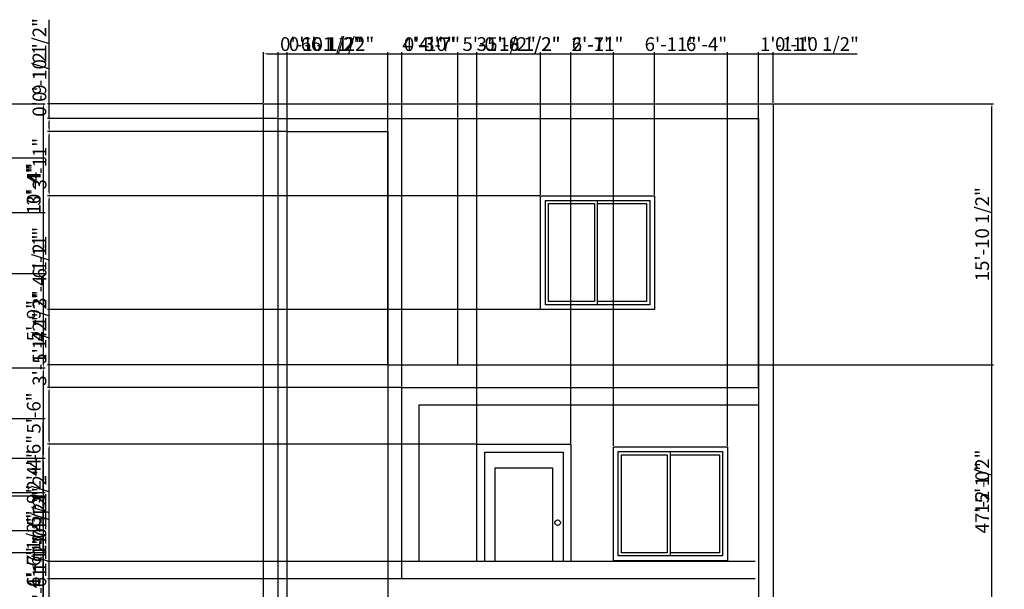
# Model space of a CAD drawing. Units: inches. Extents: x 1344 to 2521, y 3236 to 4924.
# Tile 14 of 14: x 1801 to 2521, y 4398 to 4815. Entities that reach past the tile are written whole.
import ezdxf

# ---------------------------------------------------------------- set-up
doc = ezdxf.new("R2010")
doc.units = ezdxf.units.IN
for name, color, linetype, lineweight in [('A-ANNO-DIMS', 2, 'Continuous', 18), ('A-ELEV', 7, 'Continuous', 25), ('A-GLAZ', 150, 'Continuous', 25)]:
    doc.layers.add(name, color=color, linetype=linetype, lineweight=lineweight)
doc.styles.get("Standard").update_dxf_attribs({"font": 'arial.ttf'})
doc.dimstyles.new('ISO-25', dxfattribs={"dimtxt": 10, "dimasz": 2.5, "dimexe": 1.25, "dimexo": 0.625, "dimtad": 1, "dimdec": 0, "dimlunit": 4, "dimtxsty": 'Standard', "dimcen": 2.5, "dimadec": 0, "dimazin": 0, "dimtfac": 1, "dimtdec": 0, "dimtmove": 0, "dimatfit": 3, "dimfxl": 1, "dimarcsym": 0})

# ---------------------------------------------------------------- blocks, each defined once
blk = doc.blocks.new('*U10')
for p, q in [((1.5, 1.5), (1.5, 34.5)), ((1.5, 34.5), (18, 34.5)), ((18, 1.5), (18, 34.5)), ((18, 34.5), (34.5, 34.5)), ((34.5, 34.5), (34.5, 1.5)), ((18, 1.5), (1.5, 1.5)), ((34.5, 1.5), (18, 1.5))]:
    blk.add_line(p, q)
blk.add_lwpolyline([(0, 0), (0, 36), (36, 36), (36, 0)], close=True)
for points in [[(17, 33.5), (17, 2.5), (2.5, 2.5), (2.5, 33.5), (17, 33.5)], [(18, 33.5), (33.5, 33.5), (33.5, 2.5), (18, 2.5)]]:
    blk.add_lwpolyline(points)
blk = doc.blocks.new('*D85')
at = {"layer": 'A-ANNO-DIMS', "color": 0, "lineweight": -2, "transparency": 16777216}
for p, q in [((1774.14, 4753.21), (1820.02, 4753.21)), ((1818.77, 4750.71), (1818.77, 4631.58)), ((1774.14, 4629.08), (1820.02, 4629.08))]:
    blk.add_line(p, q, dxfattribs=at)
at = {"layer": 'A-ANNO-DIMS', "color": 0, "lineweight": 100, "transparency": 16777216}
for points in [[(1818.35, 4750.71), (1819.18, 4750.71), (1818.77, 4753.21)], [(1818.35, 4631.58), (1819.18, 4631.58), (1818.77, 4629.08)]]:
    blk.add_solid(points, dxfattribs=at)
at = {"layer": 'Defpoints', "color": 0, "lineweight": 100, "transparency": 16777216}
for p in [(1773.52, 4753.21), (1773.52, 4629.08), (1818.77, 4629.08)]:
    blk.add_point(p, dxfattribs=at)
at = {"layer": 'A-ANNO-DIMS', "color": 0, "transparency": 16777216, "insert": (1813.04, 4691.15), "char_height": 10, "attachment_point": 5, "rotation": 90}
blk.add_mtext('10\'-4"', dxfattribs=at)
blk = doc.blocks.new('*D86')
at = {"layer": 'A-ANNO-DIMS', "color": 0, "lineweight": -2, "transparency": 16777216}
for p, q in [((1774.14, 4629.08), (1820.02, 4629.08)), ((1818.77, 4626.58), (1818.77, 4562.66)), ((1774.14, 4560.16), (1820.02, 4560.16))]:
    blk.add_line(p, q, dxfattribs=at)
at = {"layer": 'A-ANNO-DIMS', "color": 0, "lineweight": 100, "transparency": 16777216}
for points in [[(1818.35, 4626.58), (1819.18, 4626.58), (1818.77, 4629.08)], [(1818.35, 4562.66), (1819.18, 4562.66), (1818.77, 4560.16)]]:
    blk.add_solid(points, dxfattribs=at)
at = {"layer": 'Defpoints', "color": 0, "lineweight": 100, "transparency": 16777216}
for p in [(1773.52, 4629.08), (1773.52, 4560.16), (1818.77, 4560.16)]:
    blk.add_point(p, dxfattribs=at)
at = {"layer": 'A-ANNO-DIMS', "color": 0, "transparency": 16777216, "insert": (1813.04, 4594.62), "char_height": 10, "attachment_point": 5, "rotation": 90}
blk.add_mtext('5\'-9"', dxfattribs=at)
blk = doc.blocks.new('*D87')
at = {"layer": 'A-ANNO-DIMS', "color": 0, "lineweight": -2, "transparency": 16777216}
for p, q in [((1774.14, 4560.16), (1820.02, 4560.16)), ((1818.77, 4557.66), (1818.77, 4496.69)), ((1774.14, 4494.19), (1820.02, 4494.19))]:
    blk.add_line(p, q, dxfattribs=at)
at = {"layer": 'A-ANNO-DIMS', "color": 0, "lineweight": 100, "transparency": 16777216}
for points in [[(1818.35, 4557.66), (1819.18, 4557.66), (1818.77, 4560.16)], [(1818.35, 4496.69), (1819.18, 4496.69), (1818.77, 4494.19)]]:
    blk.add_solid(points, dxfattribs=at)
at = {"layer": 'Defpoints', "color": 0, "lineweight": 100, "transparency": 16777216}
for p in [(1773.52, 4560.16), (1773.52, 4494.19), (1818.77, 4494.19)]:
    blk.add_point(p, dxfattribs=at)
at = {"layer": 'A-ANNO-DIMS', "color": 0, "transparency": 16777216, "insert": (1813.04, 4527.17), "char_height": 10, "attachment_point": 5, "rotation": 90}
blk.add_mtext('5\'-6"', dxfattribs=at)
blk = doc.blocks.new('*D88')
at = {"layer": 'A-ANNO-DIMS', "color": 0, "lineweight": -2, "transparency": 16777216}
for p, q in [((1774.14, 4494.19), (1820.02, 4494.19)), ((1818.77, 4491.69), (1818.77, 4427.77)), ((1774.14, 4425.27), (1820.02, 4425.27))]:
    blk.add_line(p, q, dxfattribs=at)
at = {"layer": 'A-ANNO-DIMS', "color": 0, "lineweight": 100, "transparency": 16777216}
for points in [[(1818.35, 4491.69), (1819.18, 4491.69), (1818.77, 4494.19)], [(1818.35, 4427.77), (1819.18, 4427.77), (1818.77, 4425.27)]]:
    blk.add_solid(points, dxfattribs=at)
at = {"layer": 'Defpoints', "color": 0, "lineweight": 100, "transparency": 16777216}
for p in [(1773.52, 4494.19), (1773.52, 4425.27), (1818.77, 4425.27)]:
    blk.add_point(p, dxfattribs=at)
at = {"layer": 'A-ANNO-DIMS', "color": 0, "transparency": 16777216, "insert": (1813.04, 4459.73), "char_height": 10, "attachment_point": 5, "rotation": 90}
blk.add_mtext('5\'-9"', dxfattribs=at)
blk = doc.blocks.new('*D89')
at = {"layer": 'A-ANNO-DIMS', "color": 0, "lineweight": -2, "transparency": 16777216}
for p, q in [((1774.14, 4425.27), (1820.02, 4425.27)), ((1818.77, 4422.77), (1818.77, 4155.71)), ((1774.14, 4153.21), (1820.02, 4153.21))]:
    blk.add_line(p, q, dxfattribs=at)
at = {"layer": 'A-ANNO-DIMS', "color": 0, "lineweight": 100, "transparency": 16777216}
for points in [[(1818.35, 4422.77), (1819.18, 4422.77), (1818.77, 4425.27)], [(1818.35, 4155.71), (1819.18, 4155.71), (1818.77, 4153.21)]]:
    blk.add_solid(points, dxfattribs=at)
at = {"layer": 'Defpoints', "color": 0, "lineweight": 100, "transparency": 16777216}
for p in [(1773.52, 4425.27), (1773.52, 4153.21), (1818.77, 4153.21)]:
    blk.add_point(p, dxfattribs=at)
at = {"layer": 'A-ANNO-DIMS', "color": 0, "transparency": 16777216, "insert": (1813.04, 4289.24), "char_height": 10, "attachment_point": 5, "rotation": 90}
blk.add_mtext('22\'-8"', dxfattribs=at)
blk = doc.blocks.new('*D94')
at = {"layer": 'A-ANNO-DIMS', "color": 0, "lineweight": -2, "transparency": 16777216}
for p, q in [((1646.07, 4713.7), (1820.02, 4713.7)), ((1818.77, 4711.2), (1818.77, 4676.2)), ((1646.07, 4673.7), (1820.02, 4673.7))]:
    blk.add_line(p, q, dxfattribs=at)
at = {"layer": 'A-ANNO-DIMS', "color": 0, "lineweight": 100, "transparency": 16777216}
for points in [[(1818.35, 4711.2), (1819.18, 4711.2), (1818.77, 4713.7)], [(1818.35, 4676.2), (1819.18, 4676.2), (1818.77, 4673.7)]]:
    blk.add_solid(points, dxfattribs=at)
at = {"layer": 'Defpoints', "color": 0, "lineweight": 100, "transparency": 16777216}
for p in [(1645.44, 4713.7), (1645.44, 4673.7), (1818.77, 4673.7)]:
    blk.add_point(p, dxfattribs=at)
at = {"layer": 'A-ANNO-DIMS', "color": 0, "transparency": 16777216, "insert": (1813.03, 4693.7), "char_height": 10, "attachment_point": 5, "rotation": 90}
blk.add_mtext('3\'-4"', dxfattribs=at)
blk = doc.blocks.new('*D98')
at = {"layer": 'A-ANNO-DIMS', "color": 0, "lineweight": -2, "transparency": 16777216}
for p, q in [((1562.2, 4466.57), (1820.02, 4466.57)), ((1818.77, 4464.07), (1818.77, 4389.64)), ((1562.2, 4387.14), (1820.02, 4387.14))]:
    blk.add_line(p, q, dxfattribs=at)
at = {"layer": 'A-ANNO-DIMS', "color": 0, "lineweight": 100, "transparency": 16777216}
for points in [[(1818.35, 4464.07), (1819.18, 4464.07), (1818.77, 4466.57)], [(1818.35, 4389.64), (1819.18, 4389.64), (1818.77, 4387.14)]]:
    blk.add_solid(points, dxfattribs=at)
at = {"layer": 'Defpoints', "color": 0, "lineweight": 100, "transparency": 16777216}
for p in [(1561.57, 4466.57), (1561.57, 4387.14), (1818.77, 4387.14)]:
    blk.add_point(p, dxfattribs=at)
at = {"layer": 'A-ANNO-DIMS', "color": 0, "transparency": 16777216, "insert": (1812.97, 4426.85), "char_height": 10, "attachment_point": 5, "rotation": 90}
blk.add_mtext('6\'-7 1/2"', dxfattribs=at)
blk = doc.blocks.new('*D103')
at = {"layer": 'A-ANNO-DIMS', "color": 0, "lineweight": -2, "transparency": 16777216}
for p, q in [((1729.14, 4441.19), (1820.02, 4441.19)), ((1818.77, 4389.64), (1818.77, 4438.69)), ((1729.14, 4387.14), (1820.02, 4387.14))]:
    blk.add_line(p, q, dxfattribs=at)
at = {"layer": 'A-ANNO-DIMS', "color": 0, "lineweight": 100, "transparency": 16777216}
for points in [[(1818.35, 4438.69), (1819.18, 4438.69), (1818.77, 4441.19)], [(1818.35, 4389.64), (1819.18, 4389.64), (1818.77, 4387.14)]]:
    blk.add_solid(points, dxfattribs=at)
at = {"layer": 'Defpoints', "color": 0, "lineweight": 100, "transparency": 16777216}
for p in [(1728.52, 4441.19), (1818.77, 4441.19), (1728.52, 4387.14)]:
    blk.add_point(p, dxfattribs=at)
at = {"layer": 'A-ANNO-DIMS', "color": 0, "transparency": 16777216, "insert": (1813.04, 4414.17), "char_height": 10, "attachment_point": 5, "rotation": 90}
blk.add_mtext('4\'-6"', dxfattribs=at)
blk = doc.blocks.new('*D104')
at = {"layer": 'A-ANNO-DIMS', "color": 0, "lineweight": -2, "transparency": 16777216}
for p, q in [((1818.77, 4469.04), (1818.77, 4499.54)), ((1729.14, 4469.04), (1820.02, 4469.04)), ((1818.77, 4443.69), (1818.77, 4466.54)), ((1729.14, 4441.19), (1820.02, 4441.19))]:
    blk.add_line(p, q, dxfattribs=at)
at = {"layer": 'A-ANNO-DIMS', "color": 0, "lineweight": 100, "transparency": 16777216}
for points in [[(1818.35, 4466.54), (1819.18, 4466.54), (1818.77, 4469.04)], [(1818.35, 4443.69), (1819.18, 4443.69), (1818.77, 4441.19)]]:
    blk.add_solid(points, dxfattribs=at)
at = {"layer": 'Defpoints', "color": 0, "lineweight": 100, "transparency": 16777216}
for p in [(1728.52, 4469.04), (1818.77, 4469.04), (1728.52, 4441.19)]:
    blk.add_point(p, dxfattribs=at)
at = {"layer": 'A-ANNO-DIMS', "color": 0, "transparency": 16777216, "insert": (1813.12, 4485.54), "char_height": 10, "attachment_point": 5, "rotation": 90}
blk.add_mtext('2\'-4"', dxfattribs=at)
blk = doc.blocks.new('*D105')
at = {"layer": 'A-ANNO-DIMS', "color": 0, "lineweight": -2, "transparency": 16777216}
for p, q in [((1729.14, 4523.04), (1820.02, 4523.04)), ((1818.77, 4471.54), (1818.77, 4520.54)), ((1729.14, 4469.04), (1820.02, 4469.04))]:
    blk.add_line(p, q, dxfattribs=at)
at = {"layer": 'A-ANNO-DIMS', "color": 0, "lineweight": 100, "transparency": 16777216}
for points in [[(1818.35, 4520.54), (1819.18, 4520.54), (1818.77, 4523.04)], [(1818.35, 4471.54), (1819.18, 4471.54), (1818.77, 4469.04)]]:
    blk.add_solid(points, dxfattribs=at)
at = {"layer": 'Defpoints', "color": 0, "lineweight": 100, "transparency": 16777216}
for p in [(1728.52, 4523.04), (1818.77, 4523.04), (1728.52, 4469.04)]:
    blk.add_point(p, dxfattribs=at)
at = {"layer": 'A-ANNO-DIMS', "color": 0, "transparency": 16777216, "insert": (1813.04, 4496.04), "char_height": 10, "attachment_point": 5, "rotation": 90}
blk.add_mtext('4\'-6"', dxfattribs=at)
blk = doc.blocks.new('*D109')
at = {"layer": 'A-ANNO-DIMS', "color": 0, "lineweight": -2, "transparency": 16777216}
for p, q in [((1979.76, 4753.81), (1979.76, 4790.94)), ((1982.26, 4789.69), (2349.74, 4789.69)), ((2352.24, 4753.81), (2352.24, 4790.94))]:
    blk.add_line(p, q, dxfattribs=at)
at = {"layer": 'A-ANNO-DIMS', "color": 0, "lineweight": 100, "transparency": 16777216}
for points in [[(1982.26, 4790.1), (1982.26, 4789.27), (1979.76, 4789.69)], [(2349.74, 4790.1), (2349.74, 4789.27), (2352.24, 4789.69)]]:
    blk.add_solid(points, dxfattribs=at)
at = {"layer": 'Defpoints', "color": 0, "lineweight": 100, "transparency": 16777216}
for p in [(2352.24, 4789.69), (1979.76, 4753.19), (2352.24, 4753.19)]:
    blk.add_point(p, dxfattribs=at)
at = {"layer": 'A-ANNO-DIMS', "color": 0, "transparency": 16777216, "insert": (2166, 4795.48), "char_height": 10, "attachment_point": 5}
blk.add_mtext('31\'-0 1/2"', dxfattribs=at)
blk = doc.blocks.new('*D110')
at = {"layer": 'A-ANNO-DIMS', "color": 0, "lineweight": -2, "transparency": 16777216}
for p, q in [((1979.76, 4753.81), (1979.76, 4790.94)), ((1982.26, 4789.69), (1988, 4789.69)), ((1990.5, 4743.07), (1990.5, 4790.94)), ((1990.5, 4789.69), (2051.9, 4789.69))]:
    blk.add_line(p, q, dxfattribs=at)
at = {"layer": 'A-ANNO-DIMS', "color": 0, "lineweight": 100, "transparency": 16777216}
for points in [[(1982.26, 4790.1), (1982.26, 4789.27), (1979.76, 4789.69)], [(1988, 4790.1), (1988, 4789.27), (1990.5, 4789.69)]]:
    blk.add_solid(points, dxfattribs=at)
at = {"layer": 'Defpoints', "color": 0, "lineweight": 100, "transparency": 16777216}
for p in [(1990.5, 4789.69), (1979.76, 4753.19), (1990.5, 4742.45)]:
    blk.add_point(p, dxfattribs=at)
at = {"layer": 'A-ANNO-DIMS', "color": 0, "transparency": 16777216, "insert": (2022.45, 4795.48), "char_height": 10, "attachment_point": 5}
blk.add_mtext('0\'-10 1/2"', dxfattribs=at)
blk = doc.blocks.new('*D111')
at = {"layer": 'A-ANNO-DIMS', "color": 0, "lineweight": -2, "transparency": 16777216}
for p, q in [((1990.5, 4743.07), (1990.5, 4790.94)), ((1993, 4789.69), (1994.47, 4789.69)), ((1996.97, 4733.39), (1996.97, 4790.94)), ((1996.97, 4789.69), (2050.6, 4789.69))]:
    blk.add_line(p, q, dxfattribs=at)
at = {"layer": 'A-ANNO-DIMS', "color": 0, "lineweight": 100, "transparency": 16777216}
for points in [[(1993, 4790.1), (1993, 4789.27), (1990.5, 4789.69)], [(1994.47, 4790.1), (1994.47, 4789.27), (1996.97, 4789.69)]]:
    blk.add_solid(points, dxfattribs=at)
at = {"layer": 'Defpoints', "color": 0, "lineweight": 100, "transparency": 16777216}
for p in [(1996.97, 4789.69), (1990.5, 4742.45), (1996.97, 4732.77)]:
    blk.add_point(p, dxfattribs=at)
at = {"layer": 'A-ANNO-DIMS', "color": 0, "transparency": 16777216, "insert": (2025.03, 4795.48), "char_height": 10, "attachment_point": 5}
blk.add_mtext('0\'-6 1/2"', dxfattribs=at)
blk = doc.blocks.new('*D112')
at = {"layer": 'A-ANNO-DIMS', "color": 0, "lineweight": -2, "transparency": 16777216}
for p, q in [((1996.97, 4733.39), (1996.97, 4790.94)), ((1999.47, 4789.69), (2068.06, 4789.69)), ((2070.56, 4733.39), (2070.56, 4790.94))]:
    blk.add_line(p, q, dxfattribs=at)
at = {"layer": 'A-ANNO-DIMS', "color": 0, "lineweight": 100, "transparency": 16777216}
for points in [[(1999.47, 4790.1), (1999.47, 4789.27), (1996.97, 4789.69)], [(2068.06, 4790.1), (2068.06, 4789.27), (2070.56, 4789.69)]]:
    blk.add_solid(points, dxfattribs=at)
at = {"layer": 'Defpoints', "color": 0, "lineweight": 100, "transparency": 16777216}
for p in [(2070.56, 4789.69), (1996.97, 4732.77), (2070.56, 4732.77)]:
    blk.add_point(p, dxfattribs=at)
at = {"layer": 'A-ANNO-DIMS', "color": 0, "transparency": 16777216, "insert": (2033.77, 4795.48), "char_height": 10, "attachment_point": 5}
blk.add_mtext('6\'-1 1/2"', dxfattribs=at)
blk = doc.blocks.new('*D113')
at = {"layer": 'A-ANNO-DIMS', "color": 0, "lineweight": -2, "transparency": 16777216}
for p, q in [((2070.56, 4733.39), (2070.56, 4790.94)), ((2073.06, 4789.69), (2119.15, 4789.69)), ((2121.65, 4743.07), (2121.65, 4790.94))]:
    blk.add_line(p, q, dxfattribs=at)
at = {"layer": 'A-ANNO-DIMS', "color": 0, "lineweight": 100, "transparency": 16777216}
for points in [[(2073.06, 4790.1), (2073.06, 4789.27), (2070.56, 4789.69)], [(2119.15, 4790.1), (2119.15, 4789.27), (2121.65, 4789.69)]]:
    blk.add_solid(points, dxfattribs=at)
at = {"layer": 'Defpoints', "color": 0, "lineweight": 100, "transparency": 16777216}
for p in [(2121.65, 4789.69), (2121.65, 4742.45), (2070.56, 4732.77)]:
    blk.add_point(p, dxfattribs=at)
at = {"layer": 'A-ANNO-DIMS', "color": 0, "transparency": 16777216, "insert": (2096.11, 4795.42), "char_height": 10, "attachment_point": 5}
blk.add_mtext('4\'-3"', dxfattribs=at)
blk = doc.blocks.new('*D114')
at = {"layer": 'A-ANNO-DIMS', "color": 0, "lineweight": -2, "transparency": 16777216}
for p, q in [((2121.65, 4743.07), (2121.65, 4790.94)), ((2124.15, 4789.69), (2179.71, 4789.69)), ((2182.21, 4686.61), (2182.21, 4790.94))]:
    blk.add_line(p, q, dxfattribs=at)
at = {"layer": 'A-ANNO-DIMS', "color": 0, "lineweight": 100, "transparency": 16777216}
for points in [[(2124.15, 4790.1), (2124.15, 4789.27), (2121.65, 4789.69)], [(2179.71, 4790.1), (2179.71, 4789.27), (2182.21, 4789.69)]]:
    blk.add_solid(points, dxfattribs=at)
at = {"layer": 'Defpoints', "color": 0, "lineweight": 100, "transparency": 16777216}
for p in [(2182.21, 4789.69), (2121.65, 4742.45), (2182.21, 4685.98)]:
    blk.add_point(p, dxfattribs=at)
at = {"layer": 'A-ANNO-DIMS', "color": 0, "transparency": 16777216, "insert": (2151.93, 4795.48), "char_height": 10, "attachment_point": 5}
blk.add_mtext('5\'-0 1/2"', dxfattribs=at)
blk = doc.blocks.new('*D115')
at = {"layer": 'A-ANNO-DIMS', "color": 0, "lineweight": -2, "transparency": 16777216}
for p, q in [((2182.21, 4686.61), (2182.21, 4790.94)), ((2184.71, 4789.69), (2262.94, 4789.69)), ((2265.44, 4686.61), (2265.44, 4790.94))]:
    blk.add_line(p, q, dxfattribs=at)
at = {"layer": 'A-ANNO-DIMS', "color": 0, "lineweight": 100, "transparency": 16777216}
for points in [[(2184.71, 4790.1), (2184.71, 4789.27), (2182.21, 4789.69)], [(2262.94, 4790.1), (2262.94, 4789.27), (2265.44, 4789.69)]]:
    blk.add_solid(points, dxfattribs=at)
at = {"layer": 'Defpoints', "color": 0, "lineweight": 100, "transparency": 16777216}
for p in [(2265.44, 4789.69), (2182.21, 4685.98), (2265.44, 4685.98)]:
    blk.add_point(p, dxfattribs=at)
at = {"layer": 'A-ANNO-DIMS', "color": 0, "transparency": 16777216, "insert": (2223.82, 4795.42), "char_height": 10, "attachment_point": 5}
blk.add_mtext('6\'-11"', dxfattribs=at)
blk = doc.blocks.new('*D116')
at = {"layer": 'A-ANNO-DIMS', "color": 0, "lineweight": -2, "transparency": 16777216}
for p, q in [((2265.44, 4686.61), (2265.44, 4790.94)), ((2267.94, 4789.69), (2339, 4789.69)), ((2341.5, 4743.07), (2341.5, 4790.94))]:
    blk.add_line(p, q, dxfattribs=at)
at = {"layer": 'A-ANNO-DIMS', "color": 0, "lineweight": 100, "transparency": 16777216}
for points in [[(2267.94, 4790.1), (2267.94, 4789.27), (2265.44, 4789.69)], [(2339, 4790.1), (2339, 4789.27), (2341.5, 4789.69)]]:
    blk.add_solid(points, dxfattribs=at)
at = {"layer": 'Defpoints', "color": 0, "lineweight": 100, "transparency": 16777216}
for p in [(2341.5, 4789.69), (2341.5, 4742.45), (2265.44, 4685.98)]:
    blk.add_point(p, dxfattribs=at)
at = {"layer": 'A-ANNO-DIMS', "color": 0, "transparency": 16777216, "insert": (2303.47, 4795.42), "char_height": 10, "attachment_point": 5}
blk.add_mtext('6\'-4"', dxfattribs=at)
blk = doc.blocks.new('*D117')
at = {"layer": 'A-ANNO-DIMS', "color": 0, "lineweight": -2, "transparency": 16777216}
for p, q in [((2341.5, 4743.07), (2341.5, 4790.94)), ((2344, 4789.69), (2349.74, 4789.69)), ((2352.24, 4753.81), (2352.24, 4790.94)), ((2352.24, 4789.69), (2413.64, 4789.69))]:
    blk.add_line(p, q, dxfattribs=at)
at = {"layer": 'A-ANNO-DIMS', "color": 0, "lineweight": 100, "transparency": 16777216}
for points in [[(2344, 4790.1), (2344, 4789.27), (2341.5, 4789.69)], [(2349.74, 4790.1), (2349.74, 4789.27), (2352.24, 4789.69)]]:
    blk.add_solid(points, dxfattribs=at)
at = {"layer": 'Defpoints', "color": 0, "lineweight": 100, "transparency": 16777216}
for p in [(2352.24, 4789.69), (2352.24, 4753.19), (2341.5, 4742.45)]:
    blk.add_point(p, dxfattribs=at)
at = {"layer": 'A-ANNO-DIMS', "color": 0, "transparency": 16777216, "insert": (2384.19, 4795.48), "char_height": 10, "attachment_point": 5}
blk.add_mtext('0\'-10 1/2"', dxfattribs=at)
blk = doc.blocks.new('*D118')
at = {"layer": 'A-ANNO-DIMS', "color": 0, "lineweight": -2, "transparency": 16777216}
for p, q in [((2070.56, 4563.07), (2070.56, 4790.94)), ((2073.06, 4789.69), (2078.31, 4789.69)), ((2080.81, 4546.46), (2080.81, 4790.94)), ((2080.81, 4789.69), (2118.91, 4789.69))]:
    blk.add_line(p, q, dxfattribs=at)
at = {"layer": 'A-ANNO-DIMS', "color": 0, "lineweight": 100, "transparency": 16777216}
for points in [[(2073.06, 4790.1), (2073.06, 4789.27), (2070.56, 4789.69)], [(2078.31, 4790.1), (2078.31, 4789.27), (2080.81, 4789.69)]]:
    blk.add_solid(points, dxfattribs=at)
at = {"layer": 'Defpoints', "color": 0, "lineweight": 100, "transparency": 16777216}
for p in [(2080.81, 4789.69), (2070.56, 4562.45), (2080.81, 4545.84)]:
    blk.add_point(p, dxfattribs=at)
at = {"layer": 'A-ANNO-DIMS', "color": 0, "transparency": 16777216, "insert": (2101.11, 4795.42), "char_height": 10, "attachment_point": 5}
blk.add_mtext('0\'-10"', dxfattribs=at)
blk = doc.blocks.new('*D119')
at = {"layer": 'A-ANNO-DIMS', "color": 0, "lineweight": -2, "transparency": 16777216}
for p, q in [((2080.81, 4546.46), (2080.81, 4790.94)), ((2083.31, 4789.69), (2133.16, 4789.69)), ((2135.66, 4504.93), (2135.66, 4790.94))]:
    blk.add_line(p, q, dxfattribs=at)
at = {"layer": 'A-ANNO-DIMS', "color": 0, "lineweight": 100, "transparency": 16777216}
for points in [[(2083.31, 4790.1), (2083.31, 4789.27), (2080.81, 4789.69)], [(2133.16, 4790.1), (2133.16, 4789.27), (2135.66, 4789.69)]]:
    blk.add_solid(points, dxfattribs=at)
at = {"layer": 'Defpoints', "color": 0, "lineweight": 100, "transparency": 16777216}
for p in [(2135.66, 4789.69), (2080.81, 4545.84), (2135.66, 4504.31)]:
    blk.add_point(p, dxfattribs=at)
at = {"layer": 'A-ANNO-DIMS', "color": 0, "transparency": 16777216, "insert": (2108.23, 4795.31), "char_height": 10, "attachment_point": 5}
blk.add_mtext('4\'-7"', dxfattribs=at)
blk = doc.blocks.new('*D120')
at = {"layer": 'A-ANNO-DIMS', "color": 0, "lineweight": -2, "transparency": 16777216}
for p, q in [((2135.66, 4504.93), (2135.66, 4790.94)), ((2138.16, 4789.69), (2201.83, 4789.69)), ((2204.33, 4504.93), (2204.33, 4790.94))]:
    blk.add_line(p, q, dxfattribs=at)
at = {"layer": 'A-ANNO-DIMS', "color": 0, "lineweight": 100, "transparency": 16777216}
for points in [[(2138.16, 4790.1), (2138.16, 4789.27), (2135.66, 4789.69)], [(2201.83, 4790.1), (2201.83, 4789.27), (2204.33, 4789.69)]]:
    blk.add_solid(points, dxfattribs=at)
at = {"layer": 'Defpoints', "color": 0, "lineweight": 100, "transparency": 16777216}
for p in [(2204.33, 4789.69), (2135.66, 4504.31), (2204.33, 4504.31)]:
    blk.add_point(p, dxfattribs=at)
at = {"layer": 'A-ANNO-DIMS', "color": 0, "transparency": 16777216, "insert": (2169.99, 4795.48), "char_height": 10, "attachment_point": 5}
blk.add_mtext('5\'-8 1/2"', dxfattribs=at)
blk = doc.blocks.new('*D121')
at = {"layer": 'A-ANNO-DIMS', "color": 0, "lineweight": -2, "transparency": 16777216}
for p, q in [((2204.33, 4504.93), (2204.33, 4790.94)), ((2206.83, 4789.69), (2232.97, 4789.69)), ((2235.47, 4503.08), (2235.47, 4790.94))]:
    blk.add_line(p, q, dxfattribs=at)
at = {"layer": 'A-ANNO-DIMS', "color": 0, "lineweight": 100, "transparency": 16777216}
for points in [[(2206.83, 4790.1), (2206.83, 4789.27), (2204.33, 4789.69)], [(2232.97, 4790.1), (2232.97, 4789.27), (2235.47, 4789.69)]]:
    blk.add_solid(points, dxfattribs=at)
at = {"layer": 'Defpoints', "color": 0, "lineweight": 100, "transparency": 16777216}
for p in [(2235.47, 4789.69), (2204.33, 4504.31), (2235.47, 4502.46)]:
    blk.add_point(p, dxfattribs=at)
at = {"layer": 'A-ANNO-DIMS', "color": 0, "transparency": 16777216, "insert": (2219.9, 4795.33), "char_height": 10, "attachment_point": 5}
blk.add_mtext('2\'-7"', dxfattribs=at)
blk = doc.blocks.new('*D122')
at = {"layer": 'A-ANNO-DIMS', "color": 0, "lineweight": -2, "transparency": 16777216}
for p, q in [((2235.47, 4503.08), (2235.47, 4790.94)), ((2237.97, 4789.69), (2316.21, 4789.69)), ((2318.71, 4503.08), (2318.71, 4790.94))]:
    blk.add_line(p, q, dxfattribs=at)
at = {"layer": 'A-ANNO-DIMS', "color": 0, "lineweight": 100, "transparency": 16777216}
for points in [[(2237.97, 4790.1), (2237.97, 4789.27), (2235.47, 4789.69)], [(2316.21, 4790.1), (2316.21, 4789.27), (2318.71, 4789.69)]]:
    blk.add_solid(points, dxfattribs=at)
at = {"layer": 'Defpoints', "color": 0, "lineweight": 100, "transparency": 16777216}
for p in [(2318.71, 4789.69), (2235.47, 4502.46), (2318.71, 4502.46)]:
    blk.add_point(p, dxfattribs=at)
at = {"layer": 'A-ANNO-DIMS', "color": 0, "transparency": 16777216, "insert": (2277.09, 4795.42), "char_height": 10, "attachment_point": 5}
blk.add_mtext('6\'-11"', dxfattribs=at)
blk = doc.blocks.new('*D123')
at = {"layer": 'A-ANNO-DIMS', "color": 0, "lineweight": -2, "transparency": 16777216}
for p, q in [((2318.71, 4503.08), (2318.71, 4790.94)), ((2321.21, 4789.69), (2339, 4789.69)), ((2341.5, 4546.46), (2341.5, 4790.94)), ((2341.5, 4789.69), (2378.66, 4789.69))]:
    blk.add_line(p, q, dxfattribs=at)
at = {"layer": 'A-ANNO-DIMS', "color": 0, "lineweight": 100, "transparency": 16777216}
for points in [[(2321.21, 4790.1), (2321.21, 4789.27), (2318.71, 4789.69)], [(2339, 4790.1), (2339, 4789.27), (2341.5, 4789.69)]]:
    blk.add_solid(points, dxfattribs=at)
at = {"layer": 'Defpoints', "color": 0, "lineweight": 100, "transparency": 16777216}
for p in [(2341.5, 4789.69), (2341.5, 4545.84), (2318.71, 4502.46)]:
    blk.add_point(p, dxfattribs=at)
at = {"layer": 'A-ANNO-DIMS', "color": 0, "transparency": 16777216, "insert": (2361.33, 4795.33), "char_height": 10, "attachment_point": 5}
blk.add_mtext('1\'-11"', dxfattribs=at)
blk = doc.blocks.new('*D136')
at = {"layer": 'A-ANNO-DIMS', "color": 0, "lineweight": -2, "transparency": 16777216}
for p, q in [((2342.13, 4562.45), (2513.22, 4562.45)), ((2511.97, 4384.95), (2511.97, 4559.95)), ((2342.13, 4382.45), (2513.22, 4382.45))]:
    blk.add_line(p, q, dxfattribs=at)
at = {"layer": 'A-ANNO-DIMS', "color": 0, "lineweight": 100, "transparency": 16777216}
for points in [[(2511.56, 4559.95), (2512.39, 4559.95), (2511.97, 4562.45)], [(2511.56, 4384.95), (2512.39, 4384.95), (2511.97, 4382.45)]]:
    blk.add_solid(points, dxfattribs=at)
at = {"layer": 'Defpoints', "color": 0, "lineweight": 100, "transparency": 16777216}
for p in [(2341.5, 4562.45), (2511.97, 4562.45), (2341.5, 4382.45)]:
    blk.add_point(p, dxfattribs=at)
at = {"layer": 'A-ANNO-DIMS', "color": 0, "transparency": 16777216, "insert": (2506.24, 4472.45), "char_height": 10, "attachment_point": 5, "rotation": 90}
blk.add_mtext('15\'-0"', dxfattribs=at)
blk = doc.blocks.new('*D137')
at = {"layer": 'A-ANNO-DIMS', "color": 0, "lineweight": -2, "transparency": 16777216}
for p, q in [((2352.87, 4753.19), (2513.22, 4753.19)), ((2511.97, 4564.95), (2511.97, 4750.69)), ((2342.13, 4562.45), (2513.22, 4562.45))]:
    blk.add_line(p, q, dxfattribs=at)
at = {"layer": 'A-ANNO-DIMS', "color": 0, "lineweight": 100, "transparency": 16777216}
for points in [[(2511.56, 4750.69), (2512.39, 4750.69), (2511.97, 4753.19)], [(2511.56, 4564.95), (2512.39, 4564.95), (2511.97, 4562.45)]]:
    blk.add_solid(points, dxfattribs=at)
at = {"layer": 'Defpoints', "color": 0, "lineweight": 100, "transparency": 16777216}
for p in [(2352.24, 4753.19), (2511.97, 4753.19), (2341.5, 4562.45)]:
    blk.add_point(p, dxfattribs=at)
at = {"layer": 'A-ANNO-DIMS', "color": 0, "transparency": 16777216, "insert": (2506.18, 4657.82), "char_height": 10, "attachment_point": 5, "rotation": 90}
blk.add_mtext('15\'-10 1/2"', dxfattribs=at)
blk = doc.blocks.new('*D138')
at = {"layer": 'A-ANNO-DIMS', "color": 0, "lineweight": -2, "transparency": 16777216}
for p, q in [((2352.87, 4753.19), (2513.22, 4753.19)), ((2511.97, 4188.98), (2511.97, 4750.69)), ((2352.87, 4186.48), (2513.22, 4186.48))]:
    blk.add_line(p, q, dxfattribs=at)
at = {"layer": 'A-ANNO-DIMS', "color": 0, "lineweight": 100, "transparency": 16777216}
for points in [[(2511.56, 4750.69), (2512.39, 4750.69), (2511.97, 4753.19)], [(2511.56, 4188.98), (2512.39, 4188.98), (2511.97, 4186.48)]]:
    blk.add_solid(points, dxfattribs=at)
at = {"layer": 'Defpoints', "color": 0, "lineweight": 100, "transparency": 16777216}
for p in [(2352.24, 4753.19), (2511.97, 4753.19), (2352.24, 4186.48)]:
    blk.add_point(p, dxfattribs=at)
at = {"layer": 'A-ANNO-DIMS', "color": 0, "transparency": 16777216, "insert": (2506.18, 4469.83), "char_height": 10, "attachment_point": 5, "rotation": 90}
blk.add_mtext('47\'-2 1/2"', dxfattribs=at)
blk = doc.blocks.new('*D142')
at = {"layer": 'A-ANNO-DIMS', "color": 0, "lineweight": -2, "transparency": 16777216}
for p, q in [((1823.03, 4382.45), (1823.03, 4436.07)), ((1989.88, 4382.45), (1821.78, 4382.45)), ((1823.03, 4342.3), (1823.03, 4379.95)), ((2142.38, 4339.8), (1821.78, 4339.8))]:
    blk.add_line(p, q, dxfattribs=at)
at = {"layer": 'A-ANNO-DIMS', "color": 0, "lineweight": 100, "transparency": 16777216}
for points in [[(1822.61, 4379.95), (1823.44, 4379.95), (1823.03, 4382.45)], [(1822.61, 4342.3), (1823.44, 4342.3), (1823.03, 4339.8)]]:
    blk.add_solid(points, dxfattribs=at)
at = {"layer": 'Defpoints', "color": 0, "lineweight": 100, "transparency": 16777216}
for p in [(1823.03, 4382.45), (1990.5, 4382.45), (2143.01, 4339.8)]:
    blk.add_point(p, dxfattribs=at)
at = {"layer": 'A-ANNO-DIMS', "color": 0, "transparency": 16777216, "insert": (1817.23, 4410.51), "char_height": 10, "attachment_point": 5, "rotation": 90}
blk.add_mtext('3\'-6 1/2"', dxfattribs=at)
blk = doc.blocks.new('*D143')
at = {"layer": 'A-ANNO-DIMS', "color": 0, "lineweight": -2, "transparency": 16777216}
for p, q in [((1823.03, 4405.88), (1823.03, 4466.34)), ((2080.18, 4405.88), (1821.78, 4405.88)), ((1823.03, 4384.95), (1823.03, 4403.38)), ((1989.88, 4382.45), (1821.78, 4382.45))]:
    blk.add_line(p, q, dxfattribs=at)
at = {"layer": 'A-ANNO-DIMS', "color": 0, "lineweight": 100, "transparency": 16777216}
for points in [[(1822.61, 4403.38), (1823.44, 4403.38), (1823.03, 4405.88)], [(1822.61, 4384.95), (1823.44, 4384.95), (1823.03, 4382.45)]]:
    blk.add_solid(points, dxfattribs=at)
at = {"layer": 'Defpoints', "color": 0, "lineweight": 100, "transparency": 16777216}
for p in [(1823.03, 4405.88), (2080.81, 4405.88), (1990.5, 4382.45)]:
    blk.add_point(p, dxfattribs=at)
at = {"layer": 'A-ANNO-DIMS', "color": 0, "transparency": 16777216, "insert": (1817.23, 4437.36), "char_height": 10, "attachment_point": 5, "rotation": 90}
blk.add_mtext('1\'-11 1/2"', dxfattribs=at)
blk = doc.blocks.new('*D144')
at = {"layer": 'A-ANNO-DIMS', "color": 0, "lineweight": -2, "transparency": 16777216}
for p, q in [((1823.03, 4418.59), (1823.03, 4471.28)), ((2135.03, 4418.59), (1821.78, 4418.59)), ((1823.03, 4408.38), (1823.03, 4416.09)), ((2080.18, 4405.88), (1821.78, 4405.88))]:
    blk.add_line(p, q, dxfattribs=at)
at = {"layer": 'A-ANNO-DIMS', "color": 0, "lineweight": 100, "transparency": 16777216}
for points in [[(1822.61, 4416.09), (1823.44, 4416.09), (1823.03, 4418.59)], [(1822.61, 4408.38), (1823.44, 4408.38), (1823.03, 4405.88)]]:
    blk.add_solid(points, dxfattribs=at)
at = {"layer": 'Defpoints', "color": 0, "lineweight": 100, "transparency": 16777216}
for p in [(1823.03, 4418.59), (2135.66, 4418.59), (2080.81, 4405.88)]:
    blk.add_point(p, dxfattribs=at)
at = {"layer": 'A-ANNO-DIMS', "color": 0, "transparency": 16777216, "insert": (1817.23, 4446.19), "char_height": 10, "attachment_point": 5, "rotation": 90}
blk.add_mtext('1\'-0 1/2"', dxfattribs=at)
blk = doc.blocks.new('*D145')
at = {"layer": 'A-ANNO-DIMS', "color": 0, "lineweight": -2, "transparency": 16777216}
for p, q in [((2135.03, 4504.31), (1821.78, 4504.31)), ((1823.03, 4421.09), (1823.03, 4501.81)), ((2135.03, 4418.59), (1821.78, 4418.59))]:
    blk.add_line(p, q, dxfattribs=at)
at = {"layer": 'A-ANNO-DIMS', "color": 0, "lineweight": 100, "transparency": 16777216}
for points in [[(1822.61, 4501.81), (1823.44, 4501.81), (1823.03, 4504.31)], [(1822.61, 4421.09), (1823.44, 4421.09), (1823.03, 4418.59)]]:
    blk.add_solid(points, dxfattribs=at)
at = {"layer": 'Defpoints', "color": 0, "lineweight": 100, "transparency": 16777216}
for p in [(1823.03, 4504.31), (2135.66, 4504.31), (2135.66, 4418.59)]:
    blk.add_point(p, dxfattribs=at)
at = {"layer": 'A-ANNO-DIMS', "color": 0, "transparency": 16777216, "insert": (1817.23, 4461.45), "char_height": 10, "attachment_point": 5, "rotation": 90}
blk.add_mtext('7\'-1 1/2"', dxfattribs=at)
blk = doc.blocks.new('*D146')
at = {"layer": 'A-ANNO-DIMS', "color": 0, "lineweight": -2, "transparency": 16777216}
for p, q in [((1823.03, 4545.84), (1823.03, 4599.46)), ((2080.18, 4545.84), (1821.78, 4545.84)), ((1823.03, 4506.81), (1823.03, 4543.34)), ((2135.03, 4504.31), (1821.78, 4504.31))]:
    blk.add_line(p, q, dxfattribs=at)
at = {"layer": 'A-ANNO-DIMS', "color": 0, "lineweight": 100, "transparency": 16777216}
for points in [[(1822.61, 4543.34), (1823.44, 4543.34), (1823.03, 4545.84)], [(1822.61, 4506.81), (1823.44, 4506.81), (1823.03, 4504.31)]]:
    blk.add_solid(points, dxfattribs=at)
at = {"layer": 'Defpoints', "color": 0, "lineweight": 100, "transparency": 16777216}
for p in [(1823.03, 4545.84), (2080.81, 4545.84), (2135.66, 4504.31)]:
    blk.add_point(p, dxfattribs=at)
at = {"layer": 'A-ANNO-DIMS', "color": 0, "transparency": 16777216, "insert": (1817.23, 4573.9), "char_height": 10, "attachment_point": 5, "rotation": 90}
blk.add_mtext('3\'-5 1/2"', dxfattribs=at)
blk = doc.blocks.new('*D147')
at = {"layer": 'A-ANNO-DIMS', "color": 0, "lineweight": -2, "transparency": 16777216}
for p, q in [((1823.03, 4562.45), (1823.03, 4615.14)), ((2069.94, 4562.45), (1821.78, 4562.45)), ((1823.03, 4548.34), (1823.03, 4559.95)), ((2080.18, 4545.84), (1821.78, 4545.84))]:
    blk.add_line(p, q, dxfattribs=at)
at = {"layer": 'A-ANNO-DIMS', "color": 0, "lineweight": 100, "transparency": 16777216}
for points in [[(1822.61, 4559.95), (1823.44, 4559.95), (1823.03, 4562.45)], [(1822.61, 4548.34), (1823.44, 4548.34), (1823.03, 4545.84)]]:
    blk.add_solid(points, dxfattribs=at)
at = {"layer": 'Defpoints', "color": 0, "lineweight": 100, "transparency": 16777216}
for p in [(1823.03, 4562.45), (2070.56, 4562.45), (2080.81, 4545.84)]:
    blk.add_point(p, dxfattribs=at)
at = {"layer": 'A-ANNO-DIMS', "color": 0, "transparency": 16777216, "insert": (1817.23, 4590.04), "char_height": 10, "attachment_point": 5, "rotation": 90}
blk.add_mtext('1\'-4 1/2"', dxfattribs=at)
blk = doc.blocks.new('*D148')
at = {"layer": 'A-ANNO-DIMS', "color": 0, "lineweight": -2, "transparency": 16777216}
for p, q in [((1823.03, 4602.75), (1823.03, 4656.37)), ((2181.58, 4602.75), (1821.78, 4602.75)), ((1823.03, 4564.95), (1823.03, 4600.25)), ((2069.94, 4562.45), (1821.78, 4562.45))]:
    blk.add_line(p, q, dxfattribs=at)
at = {"layer": 'A-ANNO-DIMS', "color": 0, "lineweight": 100, "transparency": 16777216}
for points in [[(1822.61, 4600.25), (1823.44, 4600.25), (1823.03, 4602.75)], [(1822.61, 4564.95), (1823.44, 4564.95), (1823.03, 4562.45)]]:
    blk.add_solid(points, dxfattribs=at)
at = {"layer": 'Defpoints', "color": 0, "lineweight": 100, "transparency": 16777216}
for p in [(1823.03, 4602.75), (2182.21, 4602.75), (2070.56, 4562.45)]:
    blk.add_point(p, dxfattribs=at)
at = {"layer": 'A-ANNO-DIMS', "color": 0, "transparency": 16777216, "insert": (1817.23, 4630.81), "char_height": 10, "attachment_point": 5, "rotation": 90}
blk.add_mtext('3\'-4 1/2"', dxfattribs=at)
blk = doc.blocks.new('*D149')
at = {"layer": 'A-ANNO-DIMS', "color": 0, "lineweight": -2, "transparency": 16777216}
for p, q in [((2181.58, 4685.98), (1821.78, 4685.98)), ((1823.03, 4605.25), (1823.03, 4683.48)), ((2181.58, 4602.75), (1821.78, 4602.75))]:
    blk.add_line(p, q, dxfattribs=at)
at = {"layer": 'A-ANNO-DIMS', "color": 0, "lineweight": 100, "transparency": 16777216}
for points in [[(1822.61, 4683.48), (1823.44, 4683.48), (1823.03, 4685.98)], [(1822.61, 4605.25), (1823.44, 4605.25), (1823.03, 4602.75)]]:
    blk.add_solid(points, dxfattribs=at)
at = {"layer": 'Defpoints', "color": 0, "lineweight": 100, "transparency": 16777216}
for p in [(1823.03, 4685.98), (2182.21, 4685.98), (2182.21, 4602.75)]:
    blk.add_point(p, dxfattribs=at)
at = {"layer": 'A-ANNO-DIMS', "color": 0, "transparency": 16777216, "insert": (1817.29, 4644.36), "char_height": 10, "attachment_point": 5, "rotation": 90}
blk.add_mtext('6\'-11"', dxfattribs=at)
blk = doc.blocks.new('*D150')
at = {"layer": 'A-ANNO-DIMS', "color": 0, "lineweight": -2, "transparency": 16777216}
for p, q in [((1996.34, 4732.77), (1821.78, 4732.77)), ((1823.03, 4688.48), (1823.03, 4730.27)), ((2181.58, 4685.98), (1821.78, 4685.98))]:
    blk.add_line(p, q, dxfattribs=at)
at = {"layer": 'A-ANNO-DIMS', "color": 0, "lineweight": 100, "transparency": 16777216}
for points in [[(1822.61, 4730.27), (1823.44, 4730.27), (1823.03, 4732.77)], [(1822.61, 4688.48), (1823.44, 4688.48), (1823.03, 4685.98)]]:
    blk.add_solid(points, dxfattribs=at)
at = {"layer": 'Defpoints', "color": 0, "lineweight": 100, "transparency": 16777216}
for p in [(1823.03, 4732.77), (1996.97, 4732.77), (2182.21, 4685.98)]:
    blk.add_point(p, dxfattribs=at)
at = {"layer": 'A-ANNO-DIMS', "color": 0, "transparency": 16777216, "insert": (1817.29, 4709.37), "char_height": 10, "attachment_point": 5, "rotation": 90}
blk.add_mtext('3\'-11"', dxfattribs=at)
blk = doc.blocks.new('*D151')
at = {"layer": 'A-ANNO-DIMS', "color": 0, "lineweight": -2, "transparency": 16777216}
for p, q in [((1823.03, 4742.45), (1823.03, 4796.08)), ((1989.88, 4742.45), (1821.78, 4742.45)), ((1823.03, 4735.27), (1823.03, 4739.95)), ((1996.34, 4732.77), (1821.78, 4732.77))]:
    blk.add_line(p, q, dxfattribs=at)
at = {"layer": 'A-ANNO-DIMS', "color": 0, "lineweight": 100, "transparency": 16777216}
for points in [[(1822.61, 4739.95), (1823.44, 4739.95), (1823.03, 4742.45)], [(1822.61, 4735.27), (1823.44, 4735.27), (1823.03, 4732.77)]]:
    blk.add_solid(points, dxfattribs=at)
at = {"layer": 'Defpoints', "color": 0, "lineweight": 100, "transparency": 16777216}
for p in [(1823.03, 4742.45), (1990.5, 4742.45), (1996.97, 4732.77)]:
    blk.add_point(p, dxfattribs=at)
at = {"layer": 'A-ANNO-DIMS', "color": 0, "transparency": 16777216, "insert": (1817.23, 4770.51), "char_height": 10, "attachment_point": 5, "rotation": 90}
blk.add_mtext('0\'-9 1/2"', dxfattribs=at)
blk = doc.blocks.new('*D152')
at = {"layer": 'A-ANNO-DIMS', "color": 0, "lineweight": -2, "transparency": 16777216}
for p, q in [((1823.03, 4753.19), (1823.03, 4814.59)), ((1979.14, 4753.19), (1821.78, 4753.19)), ((1823.03, 4744.95), (1823.03, 4750.69)), ((1989.88, 4742.45), (1821.78, 4742.45))]:
    blk.add_line(p, q, dxfattribs=at)
at = {"layer": 'A-ANNO-DIMS', "color": 0, "lineweight": 100, "transparency": 16777216}
for points in [[(1822.61, 4750.69), (1823.44, 4750.69), (1823.03, 4753.19)], [(1822.61, 4744.95), (1823.44, 4744.95), (1823.03, 4742.45)]]:
    blk.add_solid(points, dxfattribs=at)
at = {"layer": 'Defpoints', "color": 0, "lineweight": 100, "transparency": 16777216}
for p in [(1823.03, 4753.19), (1979.76, 4753.19), (1990.5, 4742.45)]:
    blk.add_point(p, dxfattribs=at)
at = {"layer": 'A-ANNO-DIMS', "color": 0, "transparency": 16777216, "insert": (1817.23, 4785.14), "char_height": 10, "attachment_point": 5, "rotation": 90}
blk.add_mtext('0\'-10 1/2"', dxfattribs=at)

msp = doc.modelspace()

# ---------------------------------------------------------------- linework, layer by layer
at = {"layer": 'A-ELEV'}
for p, q in [((1979.76, 4562.45), (1979.76, 4753.19)), ((1979.76, 4753.19), (2352.24, 4753.19)), ((2352.24, 4753.19), (2352.24, 4495.2)), ((1990.5, 4562.45), (1990.5, 4742.45)), ((1990.5, 4742.45), (2341.5, 4742.45)), ((2121.65, 4562.45), (2121.65, 4742.45)), ((2341.5, 4742.45), (2341.5, 4495.2)), ((1979.76, 4382.45), (1979.76, 4562.45)), ((1990.5, 4382.45), (1990.5, 4562.45)), ((2070.56, 4562.45), (2341.5, 4562.45)), ((2341.5, 4562.45), (2341.5, 4341.36)), ((2352.24, 4562.45), (2352.24, 4341.36)), ((2080.81, 4405.88), (2080.81, 4545.84)), ((2080.81, 4545.84), (2341.5, 4545.84)), ((2093.52, 4533.12), (2341.5, 4533.12)), ((2093.52, 4418.59), (2093.52, 4533.12)), ((2339.06, 4418.59), (2093.52, 4418.59)), ((2339.06, 4405.88), (2080.81, 4405.88))]:
    msp.add_line(p, q, dxfattribs=at)
msp.add_lwpolyline([(1996.97, 4732.77), (2070.56, 4732.77), (2070.56, 4382.45), (1996.97, 4382.45)], close=True, dxfattribs=at)
for points in [[(2135.66, 4418.59), (2135.66, 4504.31), (2204.33, 4504.31), (2204.33, 4418.59)], [(2141.38, 4418.59), (2141.38, 4498.54), (2198.61, 4498.54), (2198.61, 4418.59)], [(2149.01, 4418.59), (2149.01, 4487.1), (2190.98, 4487.1), (2190.98, 4418.59)], [(2204.33, 4405.88), (2135.66, 4405.88)], [(2198.61, 4405.88), (2141.38, 4405.88)], [(2190.98, 4405.88), (2149.01, 4405.88)]]:
    msp.add_lwpolyline(points, dxfattribs=at)
msp.add_circle((2194.63, 4447.03), 2.03, dxfattribs=at)

# ---------------------------------------------------------------- block references
at = {"layer": 'A-GLAZ', "xscale": 2.312102872961218, "yscale": 2.312102872961218, "zscale": 2.312102872961218}
for p in [(2182.21, 4602.75), (2235.47, 4419.22)]:
    msp.add_blockref('*U10', p, dxfattribs=at)

# ---------------------------------------------------------------- dimensions: what is measured, and where the dimension line sits
at = {"layer": 'A-ANNO-DIMS'}
for base, p1, p2, picture, middle in [((1823.03, 4753.19), (1990.5, 4742.45), (1979.76, 4753.19), '*D152', (1817.23, 4785.14)), ((1823.03, 4742.45), (1996.97, 4732.77), (1990.5, 4742.45), '*D151', (1817.23, 4770.51)), ((1818.77, 4629.08), (1773.52, 4753.21), (1773.52, 4629.08), '*D85', (1813.04, 4691.15)), ((2511.97, 4753.19), (2341.5, 4562.45), (2352.24, 4753.19), '*D137', (2506.18, 4657.82)), ((2511.97, 4753.19), (2352.24, 4186.48), (2352.24, 4753.19), '*D138', (2506.18, 4469.83)), ((1823.03, 4732.77), (2182.21, 4685.98), (1996.97, 4732.77), '*D150', (1817.29, 4709.37)), ((1818.77, 4673.7), (1645.44, 4713.7), (1645.44, 4673.7), '*D94', (1813.03, 4693.7)), ((1823.03, 4685.98), (2182.21, 4602.75), (2182.21, 4685.98), '*D149', (1817.29, 4644.36)), ((1823.03, 4602.75), (2070.56, 4562.45), (2182.21, 4602.75), '*D148', (1817.23, 4630.81)), ((1818.77, 4560.16), (1773.52, 4629.08), (1773.52, 4560.16), '*D86', (1813.04, 4594.62)), ((1823.03, 4562.45), (2080.81, 4545.84), (2070.56, 4562.45), '*D147', (1817.23, 4590.04)), ((1823.03, 4545.84), (2135.66, 4504.31), (2080.81, 4545.84), '*D146', (1817.23, 4573.9)), ((2511.97, 4562.45), (2341.5, 4382.45), (2341.5, 4562.45), '*D136', (2506.24, 4472.45)), ((1818.77, 4494.19), (1773.52, 4560.16), (1773.52, 4494.19), '*D87', (1813.04, 4527.17)), ((1818.77, 4523.04), (1728.52, 4469.04), (1728.52, 4523.04), '*D105', (1813.04, 4496.04)), ((1818.7678, 4469.0393), (1728.5178, 4441.1901), (1728.5178, 4469.0393), '*D104', (1813.1223, 4485.5408)), ((1823.03, 4504.31), (2135.66, 4418.59), (2135.66, 4504.31), '*D145', (1817.23, 4461.45)), ((1818.77, 4425.27), (1773.52, 4494.19), (1773.52, 4425.27), '*D88', (1813.04, 4459.73)), ((1823.03, 4418.59), (2080.81, 4405.88), (2135.66, 4418.59), '*D144', (1817.23, 4446.19)), ((1818.77, 4387.14), (1561.57, 4466.57), (1561.57, 4387.14), '*D98', (1812.97, 4426.85)), ((1823.03, 4405.88), (1990.5, 4382.45), (2080.81, 4405.88), '*D143', (1817.23, 4437.36)), ((1818.7678, 4441.1901), (1728.5178, 4387.143), (1728.5178, 4441.1901), '*D103', (1813.0371, 4414.1665)), ((1823.0257, 4382.4452), (2143.0066, 4339.7965), (1990.5008, 4382.4452), '*D142', (1817.2267, 4410.5088)), ((1818.77, 4153.21), (1773.52, 4425.27), (1773.52, 4153.21), '*D89', (1813.04, 4289.24))]:
    dim = msp.add_linear_dim(base=base, p1=p1, p2=p2, angle=90, dimstyle='ISO-25', override={"dimdec": 1, "dimlfac": 1, "dimrnd": 0, "dimzin": 1, "dimdsep": 46, "dimlunit": 4, "dimfrac": 2}, dxfattribs=at)
    dim.commit()
    dim.dimension.update_dxf_attribs({"geometry": picture, "text_midpoint": middle})
for base, p1, p2, picture, middle in [((2352.24, 4789.69), (1979.76, 4753.19), (2352.24, 4753.19), '*D109', (2166, 4795.48)), ((1990.5, 4789.69), (1979.76, 4753.19), (1990.5, 4742.45), '*D110', (2022.45, 4795.48)), ((1996.97, 4789.69), (1990.5, 4742.45), (1996.97, 4732.77), '*D111', (2025.03, 4795.48)), ((2070.56, 4789.69), (1996.97, 4732.77), (2070.56, 4732.77), '*D112', (2033.77, 4795.48)), ((2182.21, 4789.69), (2121.65, 4742.45), (2182.21, 4685.98), '*D114', (2151.93, 4795.48)), ((2204.33, 4789.69), (2135.66, 4504.31), (2204.33, 4504.31), '*D120', (2169.99, 4795.48)), ((2352.24, 4789.69), (2341.5, 4742.45), (2352.24, 4753.19), '*D117', (2384.19, 4795.48)), ((2121.65, 4789.69), (2070.56, 4732.77), (2121.65, 4742.45), '*D113', (2096.11, 4795.42)), ((2080.8064, 4789.6859), (2070.563, 4562.4452), (2080.8064, 4545.835), '*D118', (2101.1074, 4795.4166)), ((2135.6567, 4789.6859), (2080.8064, 4545.835), (2135.6567, 4504.309), '*D119', (2108.2316, 4795.3109)), ((2265.44, 4789.69), (2182.21, 4685.98), (2265.44, 4685.98), '*D115', (2223.82, 4795.42)), ((2235.47, 4789.69), (2204.33, 4504.31), (2235.47, 4502.46), '*D121', (2219.9, 4795.33)), ((2318.71, 4789.69), (2235.47, 4502.46), (2318.71, 4502.46), '*D122', (2277.09, 4795.42)), ((2341.5, 4789.69), (2265.44, 4685.98), (2341.5, 4742.45), '*D116', (2303.47, 4795.42)), ((2341.5, 4789.69), (2318.71, 4502.46), (2341.5, 4545.84), '*D123', (2361.33, 4795.33))]:
    dim = msp.add_linear_dim(base=base, p1=p1, p2=p2, dimstyle='ISO-25', override={"dimdec": 1, "dimlfac": 1, "dimrnd": 0, "dimzin": 1, "dimdsep": 46, "dimlunit": 4, "dimfrac": 2}, dxfattribs=at)
    dim.commit()
    dim.dimension.update_dxf_attribs({"geometry": picture, "text_midpoint": middle})

doc.saveas('drawing.dxf')
